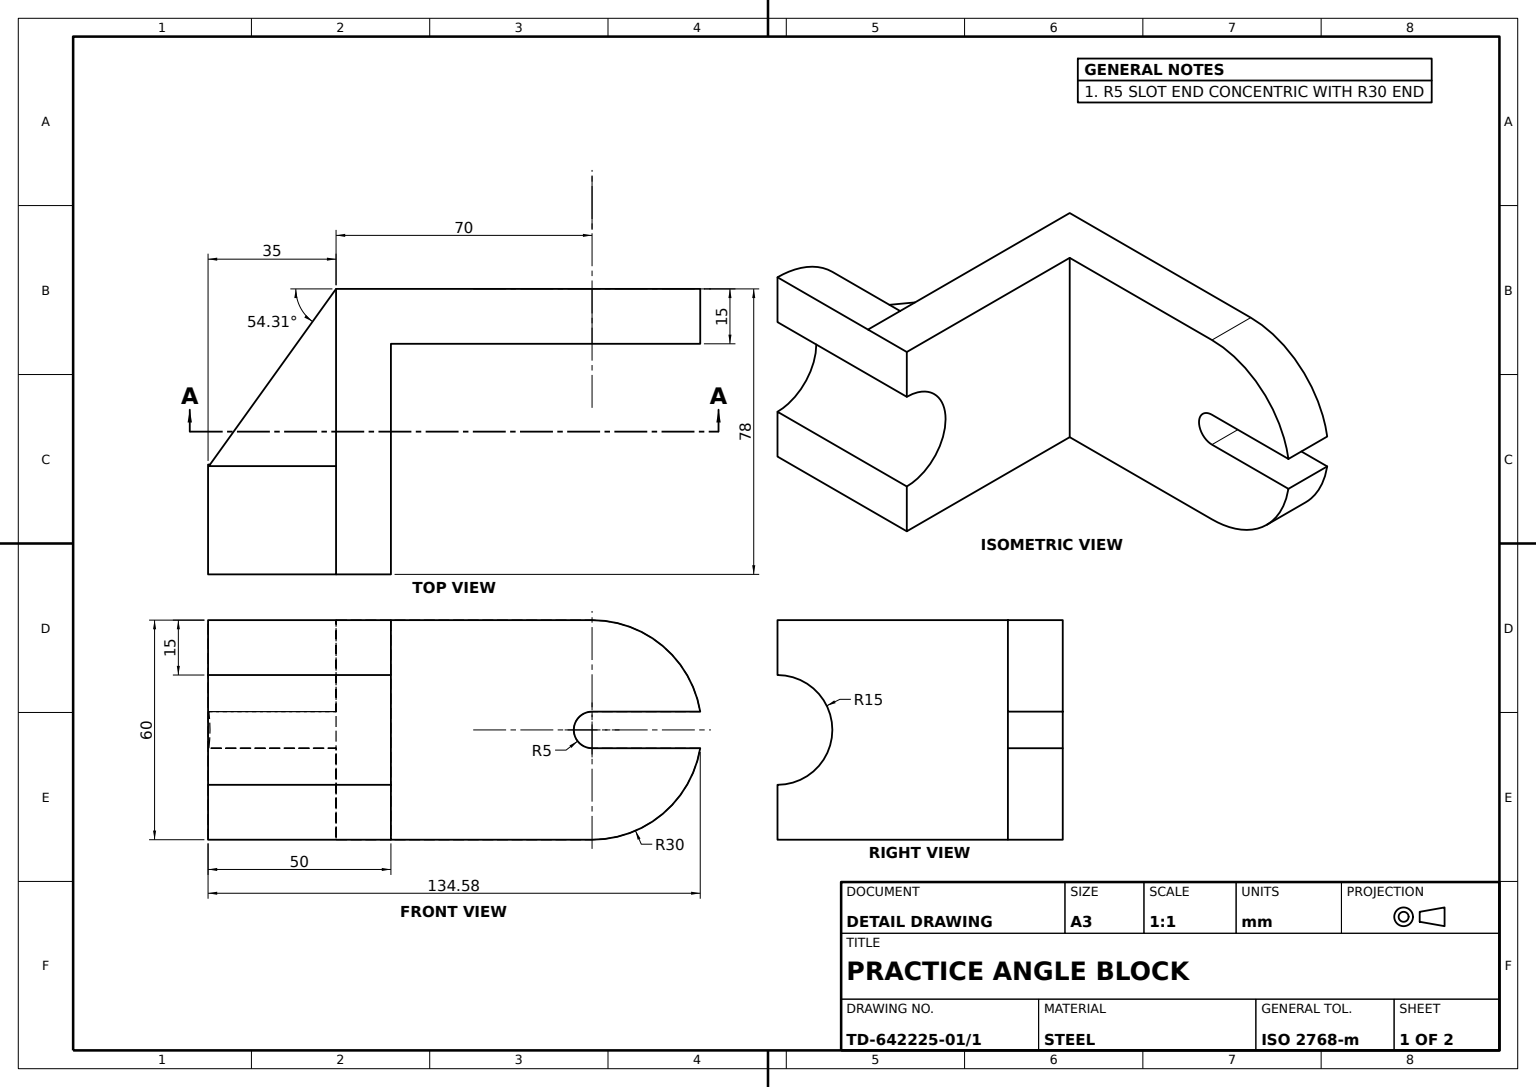
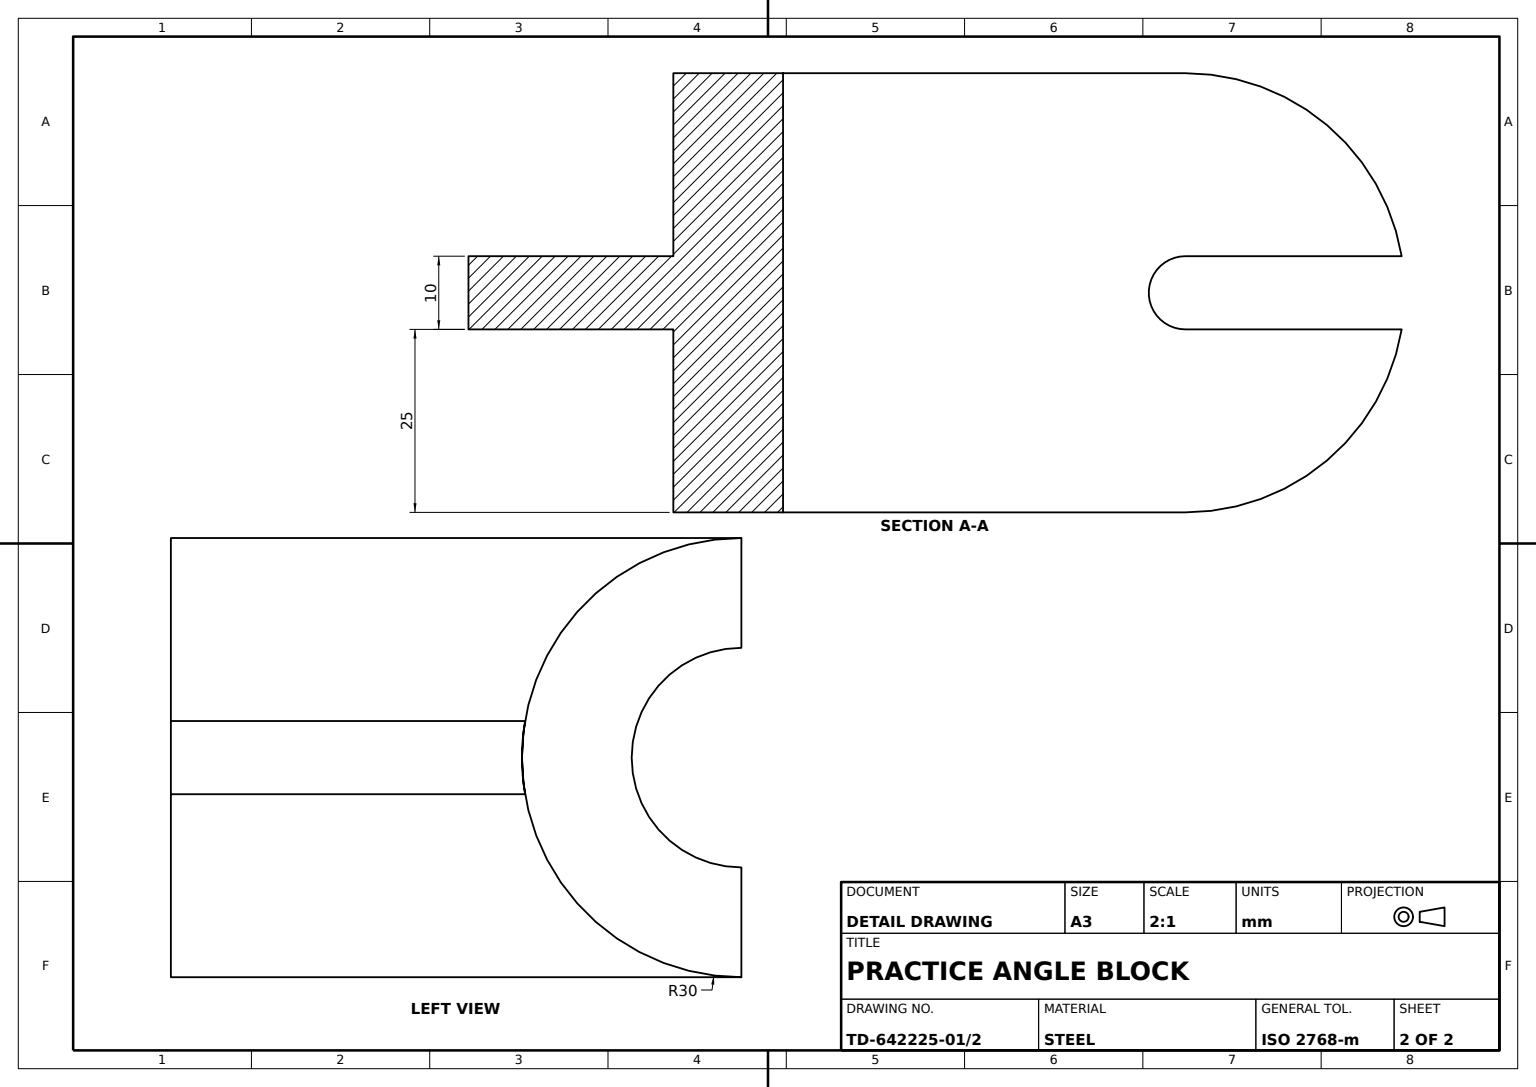
from build123d import *

# Parameters (mm, degrees)
BASE_BLOCK_SKETCH_W       = 70
BASE_BLOCK_SKETCH_H       = 60
BASE_BLOCK_60X70X15_DEPTH = 15
UPPER_ROUND_LUG_DEPTH     = 15
UPPER_SLOT_10MM_DEPTH     = 15
TOP_PLATE_SKETCH_W        = 78
TOP_PLATE_SKETCH_H        = 60
TOP_PLATE_78MM_DEPTH      = 15
RADIUS_CUT_SKETCH_R       = 30
RADIUS_CUT_DEPTH          = 15
LOWER_START               = -50
LOWER_LUG_50MM_DEPTH      = 50
SUPPORT_RIB_10MM_REACH    = 132.001
RIB_SKETCH_WALL_W         = 322.001968056
RIB_SKETCH_WALL_H         = 10


with BuildPart() as part:
    # Base Block Sketch → Base Block 60x70x15 (new body)
    with BuildSketch(Plane(origin=(0, 0, 0), x_dir=(0, 0, -1), z_dir=(1, 0, 0))):
        with Locations((35, -30)):
            Rectangle(BASE_BLOCK_SKETCH_W, BASE_BLOCK_SKETCH_H)
    extrude(amount=BASE_BLOCK_60X70X15_DEPTH)

    # Upper Lug Sketch → Upper Round Lug (add)
    with BuildSketch(Plane.ZY):
        with BuildLine():
            Line((-70, 0), (-70, -60))
            ThreePointArc((-70, -60), (-100, -30), (-70, 0))
        make_face()
    extrude(amount=-UPPER_ROUND_LUG_DEPTH)

    # Upper Slot Sketch → Upper Slot 10mm (cut)
    with BuildSketch(Plane(origin=(15, 0, 0), x_dir=(0, 0, -1), z_dir=(1, 0, 0))):
        with BuildLine():
            Line((70, -25), (99.580398915, -25))
            ThreePointArc((99.580398915, -25), (104.580398915, -30), (99.580398915, -35))
            Line((99.580398915, -35), (70, -35))
            ThreePointArc((70, -35), (65, -30), (70, -25))
        make_face()
    extrude(amount=-UPPER_SLOT_10MM_DEPTH, mode=Mode.SUBTRACT)

    # Top Plate Sketch → Top Plate 78mm (add)
    with BuildSketch(Plane.XY):
        with Locations((39, -30)):
            Rectangle(TOP_PLATE_SKETCH_W, TOP_PLATE_SKETCH_H)
    extrude(amount=-TOP_PLATE_78MM_DEPTH)

    # Radius Cut Sketch → Radius Cut (cut)
    with BuildSketch(Plane.XY):
        with Locations((78, -30)):
            Circle(RADIUS_CUT_SKETCH_R)
    extrude(amount=-RADIUS_CUT_DEPTH, mode=Mode.SUBTRACT)

    # Lower Lug Sketch → Lower Lug 50mm (add)
    with BuildSketch(Plane(origin=(0, 0, -15), x_dir=(-1, 0, 0), z_dir=(0, 0, -1)).offset(LOWER_START)):
        with BuildLine():
            Line((-78, -60), (-78, -45))
            ThreePointArc((-78, -45), (-63, -30), (-78, -15))
            Line((-78, -15), (-78, 0))
            ThreePointArc((-78, 0), (-48, -30), (-78, -60))
        make_face()
    extrude(amount=LOWER_LUG_50MM_DEPTH)

    # Rib Sketch wall → Support Rib 10mm (add, up to next)
    with BuildSketch(Plane(origin=(24.366985862, -30, 17.5), x_dir=(0.812232862067, 0, 0.583333333334), z_dir=(-0.583333333334, 0, 0.812232862067)), mode=Mode.PRIVATE) as support_rib_10mm_sk1:
        Rectangle(RIB_SKETCH_WALL_W, RIB_SKETCH_WALL_H)
    support_rib_10mm_tool1 = extrude(support_rib_10mm_sk1.sketch, amount=-SUPPORT_RIB_10MM_REACH, mode=Mode.PRIVATE) - part.part
    add(support_rib_10mm_tool1.solids().sort_by_distance((24.366985862, -30, 17.5))[0])


solid = part.part
